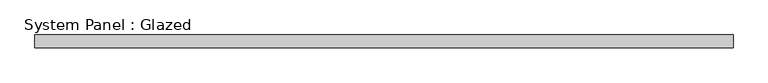
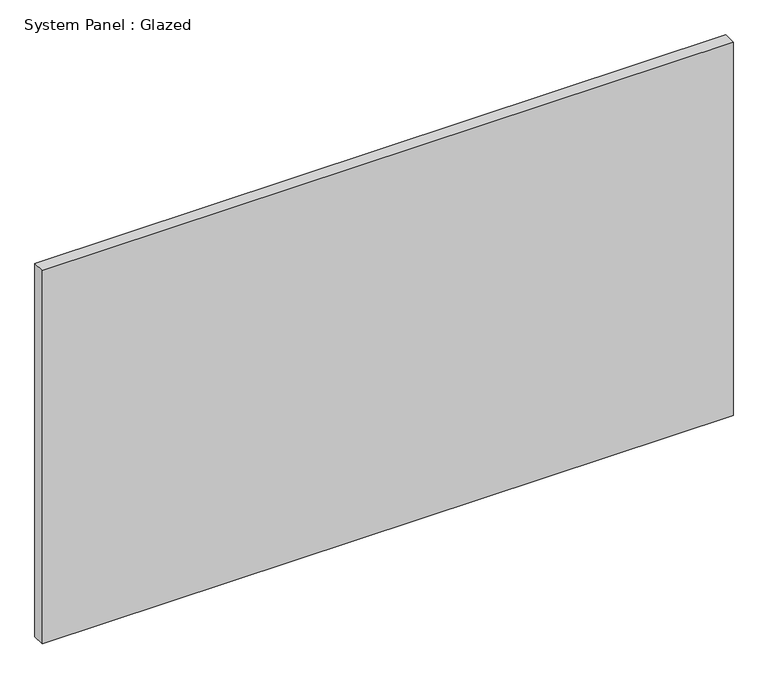
"""IFC4 building model written with IfcOpenShell, lengths in millimetres: plate geometry, System Panel : Glazed."""

from ifc_helpers import new_model, si_unit, origin, origin_with_axes, place, context, project, spatial, polyline, outline, extrude, source, transform, mapped, element, save


def system_panel_glazed_69a0d9e9(model_context):
    return source(origin(), model_context, "Body", "SweptSolid", [
        extrude(outline(polyline([(688.9750001, 19.05), (-688.9750001, 19.05), (-688.9750001, 44.45), (688.9750001, 44.45), (688.9750001, 19.05)])), origin_with_axes(), (0.0, 0.0, 1.0), 787.4),
    ])


if __name__ == "__main__":
    model = new_model("IFC4")
    model_context = context("Model", 3, world=origin())
    ifc_project = project(units=[si_unit("LENGTHUNIT", "METRE", prefix="MILLI")], contexts=[model_context])
    site = spatial("IfcSite", under=ifc_project)
    building = spatial("IfcBuilding", under=site)
    placement = place(None, origin())
    system_panel_glazed_shape = system_panel_glazed_69a0d9e9(model_context)
    element("IfcPlate", 1, ObjectType="System Panel : Glazed", at=placement, inside=building, context=model_context, shape_type="MappedRepresentation", body=[
        mapped(system_panel_glazed_shape, transform((0.0, 0.0, 0.0), x_axis=(1.0, 0.0, 0.0), y_axis=(0.0, 1.0, 0.0), z_axis=(0.0, 0.0, 1.0))),
    ])
    save(model, "model.ifc")

# Revit data of these elements
# Type "System Panel : Glazed"
#   Construction Type Id = "GSP4R"
#   Analytic Construction = "1/8 in Pilkington single glazing"
#   Visual Light Transmittance = 0.9
#   Solar Heat Gain Coefficient = 0.86
#   Heat Transfer Coefficient (U) = 1.18115 BTU/(h·ft²·°F)
#   Define Thermal Properties by = 1
# Element 1 (IfcPlate, "System Panel : Glazed")
#   Materials on its faces: "Glass"
# Materials
#   "Glass": class "Glass", colour RGB 0 128 192, transparency 0.75, Description = "Soda Lime Glass", Cost = 0
